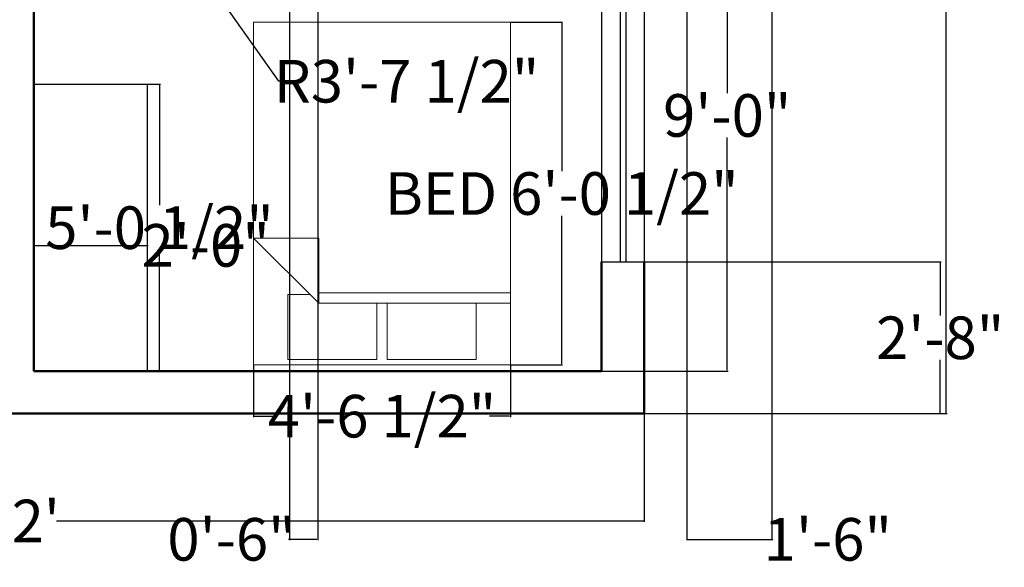
# Model space of a CAD drawing. Units: inches. Extents: x 4033 to 4435, y 499 to 1031.
# Tile 2 of 4: x 4217 to 4425, y 499 to 614. Entities that reach past the tile are written whole.
import ezdxf

# ---------------------------------------------------------------- set-up
doc = ezdxf.new("R2010")
doc.units = ezdxf.units.IN
doc.header["$MEASUREMENT"] = 0
for name, color, linetype, lineweight in [('A-ANNO-DIMS', 2, 'Continuous', 18), ('A-FLOR-CASE', 8, 'Continuous', 25), ('A-FURN', 8, 'Continuous', 18), ('A-WALL', 7, 'Continuous', 50)]:
    doc.layers.add(name, color=color, linetype=linetype, lineweight=lineweight)
doc.layers.add('A-GLAZ', color=177, linetype='Continuous', lineweight=25, true_color=0x293189)
doc.styles.get("Standard").update_dxf_attribs({"font": 'arial.ttf'})
doc.dimstyles.get("Standard").update_dxf_attribs({"dimtxt": 9, "dimasz": 0.18, "dimexe": 0.18, "dimexo": 0.0625, "dimgap": 0.09, "dimtad": 0, "dimtih": 1, "dimtoh": 1, "dimdec": 0, "dimzin": 0, "dimdsep": 46, "dimlunit": 3, "dimtxsty": 'Standard', "dimcen": 0.09, "dimadec": 0, "dimazin": 0, "dimtfac": 1, "dimtdec": 0, "dimtofl": 0, "dimtmove": 0, "dimatfit": 3, "dimfxl": 1, "dimtolj": 1, "dimtzin": 0, "dimarcsym": 0})

# ---------------------------------------------------------------- blocks, each defined once
blk = doc.blocks.new('Bed - Queen')
for p, q in [((0, -80.00003), (0, 0)), ((0, 0), (59.99999, 0)), ((59.99999, 0), (59.99999, -80.00003)), ((7.99999, -1.2), (28.79998, -1.2)), ((7.99999, -14.4), (7.99999, -1.2)), ((28.79998, -1.2), (28.79998, -14.4)), ((31.19999, -1.2), (51.99999, -1.2)), ((31.19999, -14.4), (31.19999, -1.2)), ((51.99999, -1.2), (51.99999, -16.4)), ((0, -14.4), (44.8, -14.4)), ((59.99999, -29.6), (44.8, -14.4)), ((44.8, -14.4), (44.8, -29.6)), ((44.8, -16.8), (0, -16.8)), ((51.99999, -16.4), (46.79936, -16.4)), ((44.8, -29.6), (59.99999, -29.6)), ((59.99999, -80.00003), (0, -80.00003))]:
    blk.add_line(p, q)
blk = doc.blocks.new('*D9')
at = {"layer": 'A-ANNO-DIMS', "color": 0, "lineweight": -2, "transparency": 16777216}
for p, q in [((4085.18, 531.19), (4085.18, 508.39)), ((4349.18, 531.19), (4349.18, 508.39)), ((4085.36, 508.57), (4209.37, 508.57)), ((4349, 508.57), (4224.98, 508.57))]:
    blk.add_line(p, q, dxfattribs=at)
at = {"layer": 'A-ANNO-DIMS', "color": 0, "transparency": 16777216}
for points in [[(4085.36, 508.6), (4085.36, 508.54), (4085.18, 508.57)], [(4349, 508.6), (4349, 508.54), (4349.18, 508.57)]]:
    blk.add_solid(points, dxfattribs=at)
at = {"layer": 'Defpoints', "color": 0, "transparency": 16777216}
for p in [(4085.18, 531.25), (4349.18, 531.25), (4349.18, 508.57)]:
    blk.add_point(p, dxfattribs=at)
at = {"layer": 'A-ANNO-DIMS', "color": 0, "transparency": 16777216, "insert": (4217.18, 508.57), "char_height": 9, "attachment_point": 5}
blk.add_mtext("\\A1;22'", dxfattribs=at)
blk = doc.blocks.new('*D11')
at = {"layer": 'A-ANNO-DIMS', "color": 0, "lineweight": -2, "transparency": 16777216}
for p, q in [((4305.74, 975.25), (4413.19, 975.25)), ((4413.01, 975.07), (4413.01, 757.94)), ((4413.01, 531.43), (4413.01, 748.56)), ((4349.24, 531.25), (4413.19, 531.25))]:
    blk.add_line(p, q, dxfattribs=at)
at = {"layer": 'A-ANNO-DIMS', "color": 0, "transparency": 16777216}
for points in [[(4412.98, 975.07), (4413.04, 975.07), (4413.01, 975.25)], [(4412.98, 531.43), (4413.04, 531.43), (4413.01, 531.25)]]:
    blk.add_solid(points, dxfattribs=at)
at = {"layer": 'Defpoints', "color": 0, "transparency": 16777216}
for p in [(4305.68, 975.25), (4413.01, 975.25), (4349.18, 531.25)]:
    blk.add_point(p, dxfattribs=at)
at = {"layer": 'A-ANNO-DIMS', "color": 0, "transparency": 16777216, "insert": (4413.01, 753.25), "char_height": 9, "attachment_point": 5}
blk.add_mtext("\\A1;37'", dxfattribs=at)
blk = doc.blocks.new('WIN-60IN')
for p, q in [((0, 0), (0, 9)), ((0, 9), (60, 9)), ((60, 0), (60, 9)), ((0, 5.1), (60, 5.1)), ((0, 3.9), (60, 3.9)), ((0, 0), (60, 0))]:
    blk.add_line(p, q)
blk = doc.blocks.new('*D20')
at = {"layer": 'A-ANNO-DIMS', "color": 0, "lineweight": -2, "transparency": 16777216}
for p, q in [((4320.96, 613.94), (4331.93, 613.94)), ((4331.75, 613.76), (4331.75, 582.5)), ((4331.75, 541.76), (4331.75, 573.02)), ((4320.96, 541.58), (4331.93, 541.58))]:
    blk.add_line(p, q, dxfattribs=at)
at = {"layer": 'A-ANNO-DIMS', "color": 0, "transparency": 16777216}
for points in [[(4331.72, 613.76), (4331.78, 613.76), (4331.75, 613.94)], [(4331.72, 541.76), (4331.78, 541.76), (4331.75, 541.58)]]:
    blk.add_solid(points, dxfattribs=at)
at = {"layer": 'Defpoints', "color": 0, "transparency": 16777216}
for p in [(4320.9, 613.94), (4320.9, 541.58), (4331.75, 541.58)]:
    blk.add_point(p, dxfattribs=at)
at = {"layer": 'A-ANNO-DIMS', "color": 0, "transparency": 16777216, "insert": (4331.75, 577.76), "char_height": 9, "attachment_point": 5}
blk.add_mtext('\\A1;BED 6\'-0 1/2"', dxfattribs=at)
blk = doc.blocks.new('*D21')
at = {"layer": 'A-ANNO-DIMS', "color": 0, "lineweight": -2, "transparency": 16777216}
for p, q in [((4266.62, 541.51), (4266.62, 530.54)), ((4320.9, 541.51), (4320.9, 530.54)), ((4266.8, 530.72), (4271.04, 530.72)), ((4320.72, 530.72), (4316.48, 530.72))]:
    blk.add_line(p, q, dxfattribs=at)
at = {"layer": 'A-ANNO-DIMS', "color": 0, "transparency": 16777216}
for points in [[(4266.8, 530.75), (4266.8, 530.69), (4266.62, 530.72)], [(4320.72, 530.75), (4320.72, 530.69), (4320.9, 530.72)]]:
    blk.add_solid(points, dxfattribs=at)
at = {"layer": 'Defpoints', "color": 0, "transparency": 16777216}
for p in [(4266.62, 541.58), (4320.9, 541.58), (4266.62, 530.72)]:
    blk.add_point(p, dxfattribs=at)
at = {"layer": 'A-ANNO-DIMS', "color": 0, "transparency": 16777216, "insert": (4293.76, 530.72), "char_height": 9, "attachment_point": 5}
blk.add_mtext('\\A1;4\'-6 1/2"', dxfattribs=at)
blk = doc.blocks.new('*D36')
at = {"layer": 'A-ANNO-DIMS', "color": 0, "lineweight": -2, "transparency": 16777216}
for p, q in [((4349.24, 563.3), (4411.91, 563.3)), ((4411.73, 563.12), (4411.73, 551.96)), ((4411.73, 531.43), (4411.73, 542.59)), ((4349.24, 531.25), (4411.91, 531.25))]:
    blk.add_line(p, q, dxfattribs=at)
at = {"layer": 'A-ANNO-DIMS', "color": 0, "transparency": 16777216}
for points in [[(4411.7, 563.12), (4411.76, 563.12), (4411.73, 563.3)], [(4411.7, 531.43), (4411.76, 531.43), (4411.73, 531.25)]]:
    blk.add_solid(points, dxfattribs=at)
at = {"layer": 'Defpoints', "color": 0, "transparency": 16777216}
for p in [(4349.18, 563.3), (4411.73, 563.3), (4349.18, 531.25)]:
    blk.add_point(p, dxfattribs=at)
at = {"layer": 'A-ANNO-DIMS', "color": 0, "transparency": 16777216, "insert": (4411.73, 547.28), "char_height": 9, "attachment_point": 5}
blk.add_mtext('\\A1;2\'-8"', dxfattribs=at)
blk = doc.blocks.new('*D37')
at = {"layer": 'A-ANNO-DIMS', "color": 0, "lineweight": -2, "transparency": 16777216}
for p, q in [((4340.24, 648.25), (4366.91, 648.25)), ((4366.73, 648.07), (4366.73, 598.94)), ((4366.73, 540.43), (4366.73, 589.56)), ((4340.24, 540.25), (4366.91, 540.25))]:
    blk.add_line(p, q, dxfattribs=at)
at = {"layer": 'A-ANNO-DIMS', "color": 0, "transparency": 16777216}
for points in [[(4366.7, 648.07), (4366.76, 648.07), (4366.73, 648.25)], [(4366.7, 540.43), (4366.76, 540.43), (4366.73, 540.25)]]:
    blk.add_solid(points, dxfattribs=at)
at = {"layer": 'Defpoints', "color": 0, "transparency": 16777216}
for p in [(4340.18, 648.25), (4340.18, 540.25), (4366.73, 540.25)]:
    blk.add_point(p, dxfattribs=at)
at = {"layer": 'A-ANNO-DIMS', "color": 0, "transparency": 16777216, "insert": (4366.73, 594.25), "char_height": 9, "attachment_point": 5}
blk.add_mtext('\\A1;9\'-0"', dxfattribs=at)
blk = doc.blocks.new('*D46')
at = {"layer": 'A-ANNO-DIMS', "color": 0, "lineweight": -2, "transparency": 16777216}
for p, q in [((4220.18, 540.31), (4220.18, 566.98)), ((4220.36, 566.8), (4244, 566.8)), ((4244.18, 540.31), (4244.18, 566.98)), ((4244.18, 566.8), (4244.36, 566.8))]:
    blk.add_line(p, q, dxfattribs=at)
at = {"layer": 'A-ANNO-DIMS', "color": 0, "transparency": 16777216}
for points in [[(4220.36, 566.83), (4220.36, 566.77), (4220.18, 566.8)], [(4244, 566.83), (4244, 566.77), (4244.18, 566.8)]]:
    blk.add_solid(points, dxfattribs=at)
at = {"layer": 'Defpoints', "color": 0, "transparency": 16777216}
for p in [(4244.18, 566.8), (4220.18, 540.25), (4244.18, 540.25)]:
    blk.add_point(p, dxfattribs=at)
at = {"layer": 'A-ANNO-DIMS', "color": 0, "transparency": 16777216, "insert": (4256.49, 566.8), "char_height": 9, "attachment_point": 5}
blk.add_mtext('\\A1;2\'-0"', dxfattribs=at)
blk = doc.blocks.new('*D47')
at = {"layer": 'A-ANNO-DIMS', "color": 0, "lineweight": -2, "transparency": 16777216}
for p, q in [((4220.24, 600.83), (4246.91, 600.83)), ((4246.73, 600.65), (4246.73, 575.28)), ((4246.73, 540.43), (4246.73, 565.79)), ((4220.24, 540.25), (4246.91, 540.25))]:
    blk.add_line(p, q, dxfattribs=at)
at = {"layer": 'A-ANNO-DIMS', "color": 0, "transparency": 16777216}
for points in [[(4246.7, 600.65), (4246.76, 600.65), (4246.73, 600.83)], [(4246.7, 540.43), (4246.76, 540.43), (4246.73, 540.25)]]:
    blk.add_solid(points, dxfattribs=at)
at = {"layer": 'Defpoints', "color": 0, "transparency": 16777216}
for p in [(4220.18, 600.83), (4220.18, 540.25), (4246.73, 540.25)]:
    blk.add_point(p, dxfattribs=at)
at = {"layer": 'A-ANNO-DIMS', "color": 0, "transparency": 16777216, "insert": (4246.73, 570.54), "char_height": 9, "attachment_point": 5}
blk.add_mtext('\\A1;5\'-0 1/2"', dxfattribs=at)
blk = doc.blocks.new('*D56')
at = {"layer": 'A-ANNO-DIMS', "color": 0, "lineweight": -2, "transparency": 16777216}
for p, q in [((4280.18, 654.19), (4280.18, 504.52)), ((4274.18, 648.19), (4274.18, 504.52)), ((4274.18, 504.7), (4274, 504.7)), ((4280, 504.7), (4274.36, 504.7))]:
    blk.add_line(p, q, dxfattribs=at)
at = {"layer": 'A-ANNO-DIMS', "color": 0, "transparency": 16777216}
for points in [[(4274.36, 504.73), (4274.36, 504.67), (4274.18, 504.7)], [(4280, 504.73), (4280, 504.67), (4280.18, 504.7)]]:
    blk.add_solid(points, dxfattribs=at)
at = {"layer": 'Defpoints', "color": 0, "transparency": 16777216}
for p in [(4280.18, 654.25), (4274.18, 648.25), (4274.18, 504.7)]:
    blk.add_point(p, dxfattribs=at)
at = {"layer": 'A-ANNO-DIMS', "color": 0, "transparency": 16777216, "insert": (4261.95, 504.7), "char_height": 9, "attachment_point": 5}
blk.add_mtext('\\A1;0\'-6"', dxfattribs=at)
blk = doc.blocks.new('*D59')
at = {"layer": 'A-ANNO-DIMS', "color": 0, "lineweight": -2, "transparency": 16777216}
for p, q in [((4358.18, 654.19), (4358.18, 504.52)), ((4376.18, 654.19), (4376.18, 504.52)), ((4358.36, 504.7), (4376, 504.7)), ((4376.18, 504.7), (4376.36, 504.7))]:
    blk.add_line(p, q, dxfattribs=at)
at = {"layer": 'A-ANNO-DIMS', "color": 0, "transparency": 16777216}
for points in [[(4358.36, 504.73), (4358.36, 504.67), (4358.18, 504.7)], [(4376, 504.73), (4376, 504.67), (4376.18, 504.7)]]:
    blk.add_solid(points, dxfattribs=at)
at = {"layer": 'Defpoints', "color": 0, "transparency": 16777216}
for p in [(4358.18, 654.25), (4376.18, 654.25), (4376.18, 504.7)]:
    blk.add_point(p, dxfattribs=at)
at = {"layer": 'A-ANNO-DIMS', "color": 0, "transparency": 16777216, "insert": (4387.99, 504.7), "char_height": 9, "attachment_point": 5}
blk.add_mtext('\\A1;1\'-6"', dxfattribs=at)
blk = doc.blocks.new('*D62')
at = {"layer": 'A-ANNO-DIMS', "color": 0, "lineweight": -2, "transparency": 16777216}
for p, q in [((4231.63, 658.74), (4231.81, 658.74)), ((4231.72, 658.65), (4231.72, 658.83)), ((4271.93, 601.48), (4256.96, 622.81)), ((4272.11, 601.48), (4271.93, 601.48))]:
    blk.add_line(p, q, dxfattribs=at)
at = {"layer": 'A-ANNO-DIMS', "color": 0, "transparency": 16777216}
blk.add_solid([(4256.98, 622.82), (4256.93, 622.79), (4256.85, 622.95)], dxfattribs=at)
at = {"layer": 'Defpoints', "color": 0, "transparency": 16777216}
for p in [(4231.72, 658.74), (4256.85, 622.95)]:
    blk.add_point(p, dxfattribs=at)
at = {"layer": 'A-ANNO-DIMS', "color": 0, "transparency": 16777216, "insert": (4298.96, 601.48), "char_height": 9, "attachment_point": 5}
blk.add_mtext('\\A1;R3\'-7 1/2"', dxfattribs=at)

msp = doc.modelspace()

# ---------------------------------------------------------------- linework, layer by layer
at = {"layer": 'A-FLOR-CASE'}
for p in [(4220.18, 600.83), (4244.18, 540.25)]:
    msp.add_line(p, (4244.18, 600.83), dxfattribs=at)
at = {"layer": 'A-WALL'}
for p, q in [((4220.18, 540.25), (4220.18, 645.25)), ((4340.18, 540.25), (4340.18, 563.3)), ((4349.18, 531.25), (4349.18, 563.3)), ((4220.18, 540.25), (4340.18, 540.25)), ((4208.18, 531.25), (4220.18, 531.25)), ((4220.18, 531.25), (4349.18, 531.25))]:
    msp.add_line(p, q, dxfattribs=at)

# ---------------------------------------------------------------- block references
at = {"layer": 'A-FURN', "xscale": 0.9045860936007682, "yscale": 0.9045860936007682, "zscale": 0.9045860936007682, "rotation": 180}
msp.add_blockref('Bed - Queen', (4320.9, 541.58), dxfattribs=at)
at = {"layer": 'A-GLAZ', "rotation": 270.0000000000002}
msp.add_blockref('WIN-60IN', (4340.18, 623.3), dxfattribs=at)

# ---------------------------------------------------------------- dimensions: what is measured, and where the dimension line sits
at = {"layer": 'A-ANNO-DIMS'}
for base, p1, p2, angle, override, picture, middle in [((4413.01, 975.25), (4349.18, 531.25), (4305.68, 975.25), 90, {"dimclrd": 0, "dimclre": 0, "dimclrt": 0}, '*D11', (4413.01, 753.25)), ((4366.73, 540.25), (4340.18, 648.25), (4340.18, 540.25), 270, {"dimdec": 1, "dimlfac": 1, "dimrnd": 0, "dimzin": 1, "dimdsep": 46, "dimlunit": 4, "dimfrac": 2}, '*D37', (4366.73, 594.25)), ((4246.73, 540.25), (4220.18, 600.83), (4220.18, 540.25), 270, {"dimdec": 1, "dimlfac": 1, "dimrnd": 0, "dimzin": 1, "dimdsep": 46, "dimlunit": 4, "dimfrac": 2}, '*D47', (4246.73, 570.54)), ((4411.7276, 563.3042), (4349.1776, 531.2499), (4349.1776, 563.3042), 90, {"dimdec": 1, "dimlfac": 1, "dimrnd": 0, "dimzin": 1, "dimdsep": 46, "dimlunit": 4, "dimfrac": 2}, '*D36', (4411.7276, 547.277)), ((4266.62, 530.72), (4320.9, 541.58), (4266.62, 541.58), 180, {"dimdec": 1, "dimlfac": 1, "dimrnd": 0, "dimzin": 1, "dimdsep": 46, "dimlunit": 4, "dimfrac": 2}, '*D21', (4293.76, 530.72))]:
    dim = msp.add_linear_dim(base=base, p1=p1, p2=p2, angle=angle, dimstyle='Standard', override=override, dxfattribs=at)
    dim.commit()
    dim.dimension.update_dxf_attribs({"geometry": picture, "text_midpoint": middle})
dim = msp.add_radius_dim(center=(4231.72, 658.74), mpoint=(4256.85, 622.95), dimstyle='Standard', override={"dimdec": 1, "dimlfac": 1, "dimrnd": 0, "dimzin": 1, "dimdsep": 46, "dimlunit": 4, "dimfrac": 2}, dxfattribs=at)
dim.commit()
dim.dimension.update_dxf_attribs({"geometry": '*D62', "text_midpoint": (4298.96, 601.48), "dimtype": 164})
for base, p1, p2, override, picture, middle in [((4274.18, 504.7), (4280.18, 654.25), (4274.18, 648.25), {"dimdec": 1, "dimlfac": 1, "dimrnd": 0, "dimzin": 1, "dimdsep": 46, "dimlunit": 4, "dimfrac": 2}, '*D56', (4261.95, 504.7)), ((4376.18, 504.7), (4358.18, 654.25), (4376.18, 654.25), {"dimdec": 1, "dimlfac": 1, "dimrnd": 0, "dimzin": 1, "dimdsep": 46, "dimlunit": 4, "dimfrac": 2}, '*D59', (4387.99, 504.7)), ((4244.18, 566.8), (4220.18, 540.25), (4244.18, 540.25), {"dimdec": 1, "dimlfac": 1, "dimrnd": 0, "dimzin": 1, "dimdsep": 46, "dimlunit": 4, "dimfrac": 2}, '*D46', (4256.49, 566.8)), ((4349.18, 508.57), (4085.18, 531.25), (4349.18, 531.25), {"dimclrd": 0, "dimclre": 0, "dimclrt": 0}, '*D9', (4217.18, 508.57))]:
    dim = msp.add_linear_dim(base=base, p1=p1, p2=p2, dimstyle='Standard', override=override, dxfattribs=at)
    dim.commit()
    dim.dimension.update_dxf_attribs({"geometry": picture, "text_midpoint": middle})
dim = msp.add_linear_dim(base=(4331.75, 541.58), p1=(4320.9, 613.94), p2=(4320.9, 541.58), angle=270, text='BED <>', dimstyle='Standard', override={"dimdec": 1, "dimlfac": 1, "dimrnd": 0, "dimzin": 1, "dimdsep": 46, "dimlunit": 4, "dimfrac": 2}, dxfattribs=at)
dim.commit()
dim.dimension.update_dxf_attribs({"geometry": '*D20', "text_midpoint": (4331.75, 577.76)})

doc.saveas('drawing.dxf')
